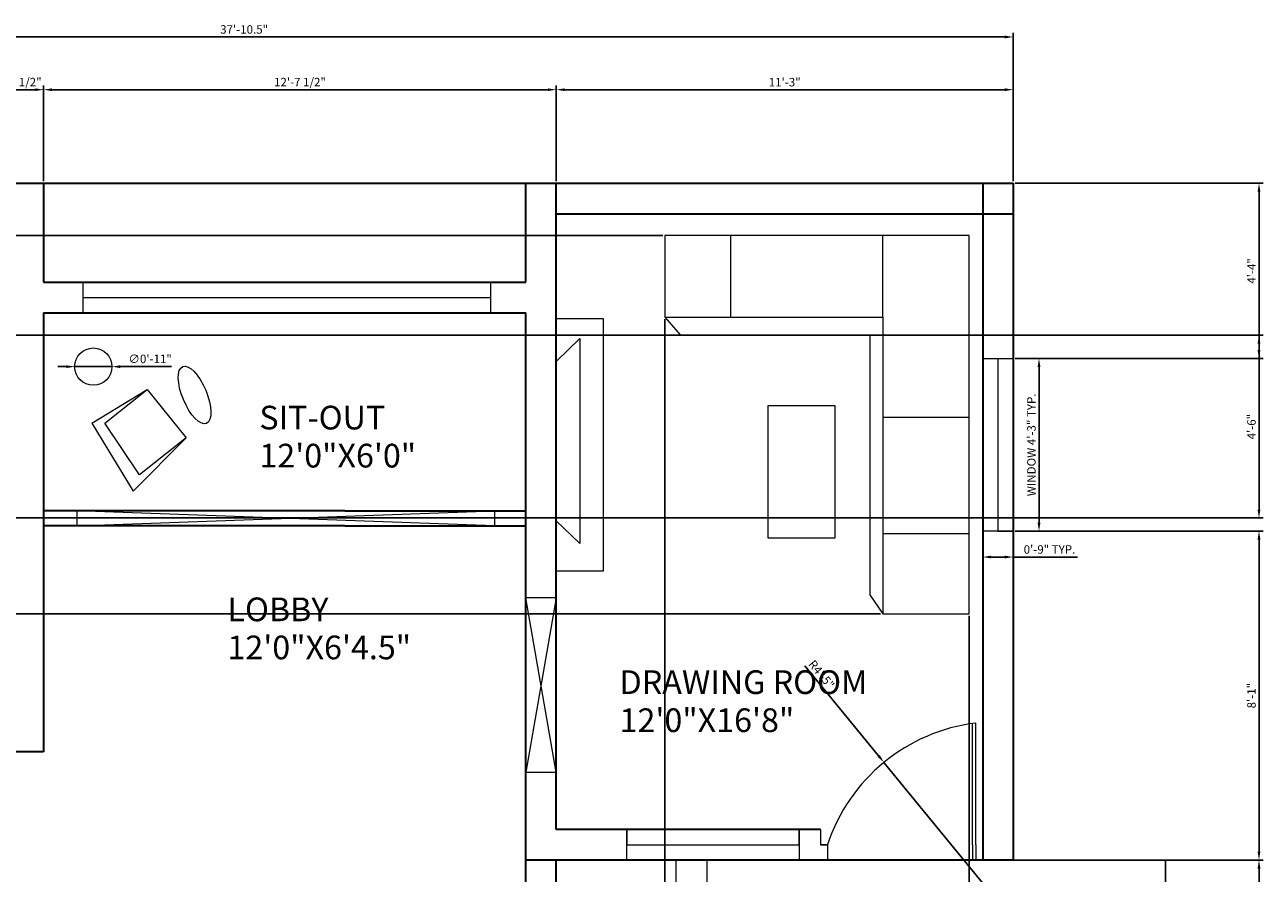
# Model space of a CAD drawing. Units: inches. Extents: x 1379 to 1989, y 1900 to 2397.
# Tile 3 of 3: x 1623 to 1989, y 2146 to 2397. Entities that reach past the tile are written whole.
import ezdxf

# ---------------------------------------------------------------- set-up
doc = ezdxf.new("R2010")
doc.units = ezdxf.units.IN
for name, color, linetype, lineweight in [('A-ANNO-DIMS', 2, 'Continuous', 18), ('A-AREA-IDEN', 7, 'Continuous', 18), ('A-DOOR', 3, 'Continuous', 18), ('A-FLOR', 7, 'Continuous', 25), ('A-FLOR-STRS', 7, 'Continuous', 18), ('A-FURN', 8, 'Continuous', 18), ('A-GLAZ', 4, 'Continuous', 18), ('A-WALL', 7, 'Continuous', 35)]:
    doc.layers.add(name, color=color, linetype=linetype, lineweight=lineweight)
doc.styles.get("Standard").update_dxf_attribs({"font": 'arial.ttf'})
doc.dimstyles.new('ISO-25', dxfattribs={"dimtxt": 2.5, "dimasz": 2.5, "dimexe": 1.25, "dimexo": 0.625, "dimtad": 1, "dimlunit": 3, "dimtxsty": 'Standard', "dimcen": 2.5, "dimadec": 0, "dimazin": 0, "dimtfac": 1, "dimtmove": 0, "dimatfit": 3, "dimfxl": 1, "dimarcsym": 0})

# ---------------------------------------------------------------- blocks, each defined once
blk = doc.blocks.new('*D6')
at = {"layer": 'A-ANNO-DIMS', "color": 0, "lineweight": -2, "transparency": 16777216}
for p, q in [((1460.41, 2350.93), (1460.41, 2394.79)), ((1462.91, 2393.54), (1912.41, 2393.54)), ((1914.91, 2350.93), (1914.91, 2394.79))]:
    blk.add_line(p, q, dxfattribs=at)
at = {"layer": 'A-ANNO-DIMS', "color": 0, "transparency": 16777216}
for points in [[(1462.91, 2393.95), (1462.91, 2393.12), (1460.41, 2393.54)], [(1912.41, 2393.95), (1912.41, 2393.12), (1914.91, 2393.54)]]:
    blk.add_solid(points, dxfattribs=at)
at = {"layer": 'Defpoints', "color": 0, "transparency": 16777216}
for p in [(1914.91, 2393.54), (1460.41, 2350.31), (1914.91, 2350.31)]:
    blk.add_point(p, dxfattribs=at)
at = {"layer": 'A-ANNO-DIMS', "color": 0, "transparency": 16777216, "insert": (1687.66, 2395.44), "char_height": 2.5, "attachment_point": 5}
blk.add_mtext('37\'-10.5"', dxfattribs=at)
blk = doc.blocks.new('WIN-51IN')
for p, q in [((0, 51), (9, 51)), ((4.5, 51), (4.5, 0)), ((9, 0), (0, 0)), ((4.5, 0), (9, 0))]:
    blk.add_line(p, q)
blk = doc.blocks.new('*D15')
at = {"layer": 'A-ANNO-DIMS', "color": 0, "lineweight": -2, "transparency": 16777216}
for p, q in [((1915.54, 2298.51), (1923.81, 2298.51)), ((1922.56, 2250.01), (1922.56, 2296.01)), ((1915.54, 2247.51), (1923.81, 2247.51))]:
    blk.add_line(p, q, dxfattribs=at)
at = {"layer": 'A-ANNO-DIMS', "color": 0, "transparency": 16777216}
for points in [[(1922.14, 2296.01), (1922.98, 2296.01), (1922.56, 2298.51)], [(1922.14, 2250.01), (1922.98, 2250.01), (1922.56, 2247.51)]]:
    blk.add_solid(points, dxfattribs=at)
at = {"layer": 'Defpoints', "color": 0, "transparency": 16777216}
for p in [(1914.91, 2298.51), (1922.56, 2298.51), (1914.91, 2247.51)]:
    blk.add_point(p, dxfattribs=at)
at = {"layer": 'A-ANNO-DIMS', "color": 0, "transparency": 16777216, "insert": (1920.64, 2273.01), "char_height": 2.5, "attachment_point": 5, "rotation": 90}
blk.add_mtext('WINDOW 4\'-3" TYP.', dxfattribs=at)
blk = doc.blocks.new('*D16')
at = {"layer": 'A-ANNO-DIMS', "color": 0, "lineweight": -2, "transparency": 16777216}
for p, q in [((1905.91, 2246.89), (1905.91, 2238.61)), ((1914.91, 2246.89), (1914.91, 2238.61)), ((1908.41, 2239.86), (1912.41, 2239.86)), ((1914.91, 2239.86), (1933.9, 2239.86))]:
    blk.add_line(p, q, dxfattribs=at)
at = {"layer": 'A-ANNO-DIMS', "color": 0, "transparency": 16777216}
for points in [[(1908.41, 2240.28), (1908.41, 2239.45), (1905.91, 2239.86)], [(1912.41, 2240.28), (1912.41, 2239.45), (1914.91, 2239.86)]]:
    blk.add_solid(points, dxfattribs=at)
at = {"layer": 'Defpoints', "color": 0, "transparency": 16777216}
for p in [(1905.91, 2247.51), (1914.91, 2247.51), (1914.91, 2239.86)]:
    blk.add_point(p, dxfattribs=at)
at = {"layer": 'A-ANNO-DIMS', "color": 0, "transparency": 16777216, "insert": (1925.65, 2241.77), "char_height": 2.5, "attachment_point": 5}
blk.add_mtext('0\'-9" TYP.', dxfattribs=at)
blk = doc.blocks.new('*D30')
at = {"layer": 'A-ANNO-DIMS', "color": 0, "lineweight": -2, "transparency": 16777216}
for p, q in [((1915.54, 2350.31), (1988.81, 2350.31)), ((1987.56, 2347.81), (1987.56, 2301.01)), ((1915.54, 2298.51), (1988.81, 2298.51))]:
    blk.add_line(p, q, dxfattribs=at)
at = {"layer": 'A-ANNO-DIMS', "color": 0, "transparency": 16777216}
for points in [[(1987.14, 2347.81), (1987.98, 2347.81), (1987.56, 2350.31)], [(1987.14, 2301.01), (1987.98, 2301.01), (1987.56, 2298.51)]]:
    blk.add_solid(points, dxfattribs=at)
at = {"layer": 'Defpoints', "color": 0, "transparency": 16777216}
for p in [(1914.91, 2350.31), (1914.91, 2298.51), (1987.56, 2298.51)]:
    blk.add_point(p, dxfattribs=at)
at = {"layer": 'A-ANNO-DIMS', "color": 0, "transparency": 16777216, "insert": (1985.69, 2324.41), "char_height": 2.5, "attachment_point": 5, "rotation": 90}
blk.add_mtext('4\'-4"', dxfattribs=at)
blk = doc.blocks.new('*D31')
at = {"layer": 'A-ANNO-DIMS', "color": 0, "lineweight": -2, "transparency": 16777216}
for p, q in [((1915.54, 2247.51), (1988.81, 2247.51)), ((1987.56, 2245.01), (1987.56, 2152.81)), ((1915.54, 2150.31), (1988.81, 2150.31))]:
    blk.add_line(p, q, dxfattribs=at)
at = {"layer": 'A-ANNO-DIMS', "color": 0, "transparency": 16777216}
for points in [[(1987.14, 2245.01), (1987.98, 2245.01), (1987.56, 2247.51)], [(1987.14, 2152.81), (1987.98, 2152.81), (1987.56, 2150.31)]]:
    blk.add_solid(points, dxfattribs=at)
at = {"layer": 'Defpoints', "color": 0, "transparency": 16777216}
for p in [(1914.91, 2247.51), (1914.91, 2150.31), (1987.56, 2150.31)]:
    blk.add_point(p, dxfattribs=at)
at = {"layer": 'A-ANNO-DIMS', "color": 0, "transparency": 16777216, "insert": (1985.66, 2198.91), "char_height": 2.5, "attachment_point": 5, "rotation": 90}
blk.add_mtext('8\'-1"', dxfattribs=at)
blk = doc.blocks.new('*D32')
at = {"layer": 'A-ANNO-DIMS', "color": 0, "lineweight": -2, "transparency": 16777216}
for p, q in [((1960.54, 2150.31), (1988.81, 2150.31)), ((1987.56, 1944.61), (1987.56, 2147.81)), ((1960.54, 1942.11), (1988.81, 1942.11))]:
    blk.add_line(p, q, dxfattribs=at)
at = {"layer": 'A-ANNO-DIMS', "color": 0, "transparency": 16777216}
for points in [[(1987.14, 2147.81), (1987.98, 2147.81), (1987.56, 2150.31)], [(1987.14, 1944.61), (1987.98, 1944.61), (1987.56, 1942.11)]]:
    blk.add_solid(points, dxfattribs=at)
at = {"layer": 'Defpoints', "color": 0, "transparency": 16777216}
for p in [(1959.91, 2150.31), (1987.56, 2150.31), (1959.91, 1942.11)]:
    blk.add_point(p, dxfattribs=at)
at = {"layer": 'A-ANNO-DIMS', "color": 0, "transparency": 16777216, "insert": (1985.68, 2046.21), "char_height": 2.5, "attachment_point": 5, "rotation": 90}
blk.add_mtext('17\'-4"', dxfattribs=at)
blk = doc.blocks.new('*D35')
at = {"layer": 'A-ANNO-DIMS', "color": 0, "lineweight": -2, "transparency": 16777216}
for p, q in [((1613.78, 2350.93), (1613.78, 2379.21)), ((1628.41, 2350.93), (1628.41, 2379.21)), ((1616.28, 2377.96), (1625.91, 2377.96))]:
    blk.add_line(p, q, dxfattribs=at)
at = {"layer": 'A-ANNO-DIMS', "color": 0, "transparency": 16777216}
for points in [[(1616.28, 2378.37), (1616.28, 2377.54), (1613.78, 2377.96)], [(1625.91, 2378.37), (1625.91, 2377.54), (1628.41, 2377.96)]]:
    blk.add_solid(points, dxfattribs=at)
at = {"layer": 'Defpoints', "color": 0, "transparency": 16777216}
for p in [(1628.41, 2377.96), (1613.78, 2350.31), (1628.41, 2350.31)]:
    blk.add_point(p, dxfattribs=at)
at = {"layer": 'A-ANNO-DIMS', "color": 0, "transparency": 16777216, "insert": (1621.1, 2379.88), "char_height": 2.5, "attachment_point": 5}
blk.add_mtext('1\'-2 1/2"', dxfattribs=at)
blk = doc.blocks.new('*D36')
at = {"layer": 'A-ANNO-DIMS', "color": 0, "lineweight": -2, "transparency": 16777216}
for p, q in [((1628.41, 2350.93), (1628.41, 2379.21)), ((1779.91, 2350.93), (1779.91, 2379.21)), ((1630.91, 2377.96), (1777.41, 2377.96))]:
    blk.add_line(p, q, dxfattribs=at)
at = {"layer": 'A-ANNO-DIMS', "color": 0, "transparency": 16777216}
for points in [[(1630.91, 2378.37), (1630.91, 2377.54), (1628.41, 2377.96)], [(1777.41, 2378.37), (1777.41, 2377.54), (1779.91, 2377.96)]]:
    blk.add_solid(points, dxfattribs=at)
at = {"layer": 'Defpoints', "color": 0, "transparency": 16777216}
for p in [(1779.91, 2377.96), (1628.41, 2350.31), (1779.91, 2350.31)]:
    blk.add_point(p, dxfattribs=at)
at = {"layer": 'A-ANNO-DIMS', "color": 0, "transparency": 16777216, "insert": (1704.16, 2379.88), "char_height": 2.5, "attachment_point": 5}
blk.add_mtext('12\'-7 1/2"', dxfattribs=at)
blk = doc.blocks.new('*D37')
at = {"layer": 'A-ANNO-DIMS', "color": 0, "lineweight": -2, "transparency": 16777216}
for p, q in [((1779.91, 2350.93), (1779.91, 2379.21)), ((1914.91, 2350.93), (1914.91, 2379.21)), ((1782.41, 2377.96), (1912.41, 2377.96))]:
    blk.add_line(p, q, dxfattribs=at)
at = {"layer": 'A-ANNO-DIMS', "color": 0, "transparency": 16777216}
for points in [[(1782.41, 2378.37), (1782.41, 2377.54), (1779.91, 2377.96)], [(1912.41, 2378.37), (1912.41, 2377.54), (1914.91, 2377.96)]]:
    blk.add_solid(points, dxfattribs=at)
at = {"layer": 'Defpoints', "color": 0, "transparency": 16777216}
for p in [(1914.91, 2377.96), (1779.91, 2350.31), (1914.91, 2350.31)]:
    blk.add_point(p, dxfattribs=at)
at = {"layer": 'A-ANNO-DIMS', "color": 0, "transparency": 16777216, "insert": (1847.41, 2379.86), "char_height": 2.5, "attachment_point": 5}
blk.add_mtext('11\'-3"', dxfattribs=at)
blk = doc.blocks.new('*D41')
at = {"layer": 'A-ANNO-DIMS', "color": 0, "lineweight": -2, "transparency": 16777216}
for p, q in [((1548.89, 2305.4), (1988.81, 2305.4)), ((1987.56, 2302.9), (1987.56, 2253.9)), ((1548.89, 2251.4), (1988.81, 2251.4))]:
    blk.add_line(p, q, dxfattribs=at)
at = {"layer": 'A-ANNO-DIMS', "color": 0, "transparency": 16777216}
for points in [[(1987.14, 2302.9), (1987.98, 2302.9), (1987.56, 2305.4)], [(1987.14, 2253.9), (1987.98, 2253.9), (1987.56, 2251.4)]]:
    blk.add_solid(points, dxfattribs=at)
at = {"layer": 'Defpoints', "color": 0, "transparency": 16777216}
for p in [(1548.27, 2305.4), (1548.27, 2251.4), (1987.56, 2251.4)]:
    blk.add_point(p, dxfattribs=at)
at = {"layer": 'A-ANNO-DIMS', "color": 0, "transparency": 16777216, "insert": (1985.66, 2278.4), "char_height": 2.5, "attachment_point": 5, "rotation": 90}
blk.add_mtext('4\'-6"', dxfattribs=at)
blk = doc.blocks.new('*D42')
at = {"layer": 'A-ANNO-DIMS', "color": 0, "lineweight": -2, "transparency": 16777216}
for p, q in [((1811.97, 2310.14), (1811.97, 1900.58)), ((1901.92, 2222.46), (1901.92, 1900.58)), ((1814.47, 1901.83), (1899.42, 1901.83))]:
    blk.add_line(p, q, dxfattribs=at)
at = {"layer": 'A-ANNO-DIMS', "color": 0, "transparency": 16777216}
for points in [[(1814.47, 1902.24), (1814.47, 1901.41), (1811.97, 1901.83)], [(1899.42, 1902.24), (1899.42, 1901.41), (1901.92, 1901.83)]]:
    blk.add_solid(points, dxfattribs=at)
at = {"layer": 'Defpoints', "color": 0, "transparency": 16777216}
for p in [(1811.97, 2310.77), (1901.92, 2223.09), (1901.92, 1901.83)]:
    blk.add_point(p, dxfattribs=at)
at = {"layer": 'A-ANNO-DIMS', "color": 0, "transparency": 16777216, "insert": (1856.94, 1903.73), "char_height": 2.5, "attachment_point": 5}
blk.add_mtext('7\'-6"', dxfattribs=at)
blk = doc.blocks.new('*D43')
at = {"layer": 'A-ANNO-DIMS', "color": 0, "lineweight": -2, "transparency": 16777216}
for p, q in [((1811.35, 2334.84), (1380.86, 2334.84)), ((1382.11, 2332.34), (1382.11, 2225.59)), ((1875.73, 2223.09), (1380.86, 2223.09))]:
    blk.add_line(p, q, dxfattribs=at)
at = {"layer": 'A-ANNO-DIMS', "color": 0, "transparency": 16777216}
for points in [[(1381.7, 2332.34), (1382.53, 2332.34), (1382.11, 2334.84)], [(1381.7, 2225.59), (1382.53, 2225.59), (1382.11, 2223.09)]]:
    blk.add_solid(points, dxfattribs=at)
at = {"layer": 'Defpoints', "color": 0, "transparency": 16777216}
for p in [(1811.97, 2334.84), (1382.11, 2223.09), (1876.36, 2223.09)]:
    blk.add_point(p, dxfattribs=at)
at = {"layer": 'A-ANNO-DIMS', "color": 0, "transparency": 16777216, "insert": (1380.21, 2278.96), "char_height": 2.5, "attachment_point": 5, "rotation": 90}
blk.add_mtext('9\'-4"', dxfattribs=at)
blk = doc.blocks.new('*D44')
at = {"layer": 'A-ANNO-DIMS', "color": 0, "lineweight": -2, "transparency": 16777216}
for p, q in [((1853.31, 2207.74), (1875.14, 2181.12)), ((1910.32, 2138.22), (1876.73, 2179.19))]:
    blk.add_line(p, q, dxfattribs=at)
at = {"layer": 'A-ANNO-DIMS', "color": 0, "transparency": 16777216}
blk.add_solid([(1875.47, 2181.38), (1874.82, 2180.85), (1876.73, 2179.19)], dxfattribs=at)
at = {"layer": 'Defpoints', "color": 0, "transparency": 16777216}
for p in [(1876.73, 2179.19), (1910.32, 2138.22)]:
    blk.add_point(p, dxfattribs=at)
at = {"layer": 'A-ANNO-DIMS', "color": 0, "transparency": 16777216, "insert": (1858.04, 2204.97), "char_height": 2.5, "attachment_point": 5, "rotation": 309.3523}
blk.add_mtext('R4\'-5"', dxfattribs=at)
blk = doc.blocks.new('*D51')
at = {"layer": 'A-ANNO-DIMS', "color": 0, "lineweight": -2, "transparency": 16777216}
for p, q in [((1635.07, 2296.12), (1632.57, 2296.12)), ((1637.57, 2296.12), (1648.6, 2296.12)), ((1666.16, 2296.12), (1651.1, 2296.12))]:
    blk.add_line(p, q, dxfattribs=at)
at = {"layer": 'A-ANNO-DIMS', "color": 0, "transparency": 16777216}
for points in [[(1635.07, 2296.54), (1635.07, 2295.7), (1637.57, 2296.12)], [(1651.1, 2296.54), (1651.1, 2295.7), (1648.6, 2296.12)]]:
    blk.add_solid(points, dxfattribs=at)
at = {"layer": 'Defpoints', "color": 0, "transparency": 16777216}
for p in [(1637.57, 2296.12), (1648.6, 2296.12)]:
    blk.add_point(p, dxfattribs=at)
at = {"layer": 'A-ANNO-DIMS', "color": 0, "transparency": 16777216, "insert": (1659.88, 2298.09), "char_height": 2.5, "attachment_point": 5, "rotation": 0.003}
blk.add_mtext('∅0\'-11"', dxfattribs=at)

msp = doc.modelspace()

# ---------------------------------------------------------------- linework, layer by layer
at = {"layer": 'A-DOOR'}
for p, q in [((1902.91, 2154.808), (1902.91, 2190.676)), ((1903.91, 2154.808), (1903.91, 2190.808)), ((1858.009, 2159.308), (1858.009, 2154.808)), ((1905.91, 2159.308), (1905.91, 2154.808)), ((1858.009, 2154.808), (1860.009, 2154.808)), ((1860.009, 2154.808), (1858.009, 2154.808)), ((1860.009, 2154.808), (1860.009, 2150.308)), ((1902.91, 2154.808), (1902.91, 2150.308)), ((1903.91, 2154.808), (1903.91, 2150.308))]:
    msp.add_line(p, q, dxfattribs=at)
msp.add_arc((1910.322, 2138.221), 52.977, 96.95114, 161.75354, dxfattribs=at)
at = {"layer": 'A-FLOR'}
for p, q in [((1959.91, 2150.308), (1914.91, 2150.308)), ((1959.91, 2049.582), (1959.91, 2150.308))]:
    msp.add_line(p, q, dxfattribs=at)
at = {"layer": 'A-FLOR-STRS'}
for p, q in [((1815.368, 2046.02), (1815.368, 2150.308)), ((1824.368, 2150.308), (1824.368, 2045.838))]:
    msp.add_line(p, q, dxfattribs=at)
at = {"layer": 'A-FURN'}
for p, q in [((1811.97, 2334.839), (1811.97, 2310.77)), ((1901.918, 2334.839), (1811.97, 2334.839)), ((1831.376, 2334.839), (1831.376, 2310.77)), ((1876.359, 2310.77), (1876.359, 2334.839)), ((1901.918, 2223.089), (1901.918, 2334.839)), ((1779.91, 2310.332), (1793.758, 2310.332)), ((1793.758, 2310.332), (1793.758, 2235.684)), ((1811.97, 2310.77), (1876.359, 2310.77)), ((1811.97, 2310.77), (1816.463, 2305.541)), ((1831.376, 2310.77), (1876.359, 2310.77)), ((1876.359, 2310.77), (1876.359, 2223.089)), ((1779.91, 2297.612), (1786.829, 2304.448)), ((1786.829, 2304.448), (1786.829, 2243.831)), ((1816.463, 2305.541), (1872.587, 2305.541)), ((1872.587, 2305.541), (1872.587, 2228.737)), ((1642.639, 2279.436), (1659.035, 2289.416)), ((1646.514, 2279.436), (1659.035, 2289.416)), ((1659.035, 2289.416), (1670.494, 2275.041)), ((1876.359, 2281.159), (1901.918, 2281.159)), ((1642.639, 2279.436), (1654.881, 2259.324)), ((1656.782, 2264.111), (1646.514, 2279.436)), ((1654.881, 2259.324), (1670.494, 2275.041)), ((1670.494, 2275.041), (1656.782, 2264.111)), ((1786.829, 2243.831), (1779.91, 2250.56)), ((1876.359, 2246.795), (1901.918, 2246.795)), ((1793.758, 2235.684), (1779.91, 2235.684)), ((1872.587, 2228.737), (1876.359, 2223.089)), ((1876.359, 2223.089), (1901.918, 2223.089))]:
    msp.add_line(p, q, dxfattribs=at)
msp.add_lwpolyline([(1842.556, 2284.681), (1862.194, 2284.681), (1862.194, 2245.428), (1842.556, 2245.428)], close=True, dxfattribs=at)
msp.add_circle((1643.086, 2296.12), 5.515, dxfattribs=at)
msp.add_ellipse((1673.02, 2287.75), major_axis=(3.501, -8.385), ratio=0.3949454, dxfattribs=at)
at = {"layer": 'A-GLAZ'}
for p, q in [((1639.98, 2321.038), (1639.98, 2312.038)), ((1760.445, 2321.038), (1760.445, 2312.038)), ((1639.98, 2316.538), (1760.445, 2316.538)), ((1638.173, 2253.538), (1638.173, 2249.038)), ((1638.173, 2249.038), (1761.604, 2253.538)), ((1761.604, 2249.038), (1638.173, 2253.538)), ((1761.604, 2253.538), (1761.604, 2249.038)), ((1779.91, 2227.839), (1770.91, 2227.839)), ((1779.91, 2227.839), (1770.91, 2176.31)), ((1779.91, 2176.31), (1770.91, 2227.839)), ((1770.91, 2176.31), (1779.91, 2176.31)), ((1770.91, 2176.31), (1779.91, 2176.31)), ((1800.714, 2159.308), (1800.714, 2154.808))]:
    msp.add_line(p, q, dxfattribs=at)
at = {"layer": 'A-WALL'}
for p, q in [((1460.41, 2350.308), (1628.41, 2350.308)), ((1628.41, 2350.308), (1628.41, 2321.038)), ((1628.41, 2350.308), (1760.41, 2350.308)), ((1760.41, 2350.308), (1779.91, 2350.308)), ((1770.91, 2350.308), (1914.91, 2350.308)), ((1770.91, 2321.038), (1770.91, 2350.308)), ((1779.91, 2159.308), (1779.91, 2350.308)), ((1905.91, 2350.308), (1905.91, 2150.308)), ((1914.91, 2350.308), (1914.91, 2150.308)), ((1779.91, 2341.308), (1914.91, 2341.308)), ((1628.41, 2321.038), (1770.91, 2321.038)), ((1628.41, 2312.038), (1770.91, 2312.038)), ((1628.41, 2312.038), (1628.41, 2182.308)), ((1770.91, 2040.582), (1770.91, 2312.038)), ((1717.462, 2253.538), (1628.41, 2253.538)), ((1717.462, 2253.538), (1770.91, 2253.538)), ((1717.462, 2249.038), (1628.41, 2249.038)), ((1717.462, 2249.038), (1770.91, 2249.038)), ((1628.41, 2182.308), (1613.41, 2182.308)), ((1858.009, 2159.308), (1779.91, 2159.308)), ((1914.91, 2150.308), (1770.91, 2150.308)), ((1779.91, 2049.582), (1779.91, 2150.308))]:
    msp.add_line(p, q, dxfattribs=at)

# ---------------------------------------------------------------- block references
at = {"layer": 'A-GLAZ'}
msp.add_blockref('WIN-51IN', (1905.91, 2247.514), dxfattribs=at)
at = {"layer": 'A-GLAZ', "rotation": 89.99999999999955}
msp.add_blockref('WIN-51IN', (1851.715, 2150.308), dxfattribs=at)

# ---------------------------------------------------------------- texts
at = {"layer": 'A-AREA-IDEN'}
for s, p in [('SIT-OUT', (1692.153, 2277.567)), ('12\'0"X6\'0"', (1692.153, 2266.322)), ('LOBBY', (1682.716, 2220.9)), ('12\'0"X6\'4.5"', (1682.716, 2209.656)), ('DRAWING ROOM', (1798.594, 2199.391)), ('12\'0"X16\'8"', (1798.594, 2188.146))]:
    msp.add_text(s, height=7, dxfattribs=at).set_placement(p)

# ---------------------------------------------------------------- dimensions: what is measured, and where the dimension line sits
at = {"layer": 'A-ANNO-DIMS'}
for base, p1, p2, override, picture, middle in [((1914.91, 2393.536), (1460.41, 2350.308), (1914.91, 2350.308), {"dimclrd": 0, "dimclre": 0, "dimclrt": 0}, '*D6', (1687.66, 2395.438)), ((1628.41, 2377.958), (1613.78, 2350.308), (1628.41, 2350.308), {"dimdec": 1, "dimlfac": 1, "dimrnd": 0, "dimzin": 1, "dimdsep": 46, "dimlunit": 4, "dimfrac": 2}, '*D35', (1621.095, 2379.875)), ((1779.91, 2377.958), (1628.41, 2350.308), (1779.91, 2350.308), {"dimdec": 1, "dimlfac": 1, "dimrnd": 0, "dimzin": 1, "dimdsep": 46, "dimlunit": 4, "dimfrac": 2}, '*D36', (1704.16, 2379.875)), ((1914.91, 2377.958), (1779.91, 2350.308), (1914.91, 2350.308), {"dimdec": 1, "dimlfac": 1, "dimrnd": 0, "dimzin": 1, "dimdsep": 46, "dimlunit": 4, "dimfrac": 2}, '*D37', (1847.41, 2379.86)), ((1901.918, 1901.828), (1811.97, 2310.77), (1901.918, 2223.089), {"dimdec": 1, "dimlfac": 1, "dimrnd": 0, "dimzin": 1, "dimdsep": 46, "dimlunit": 4, "dimfrac": 2}, '*D42', (1856.944, 1903.729))]:
    dim = msp.add_linear_dim(base=base, p1=p1, p2=p2, dimstyle='ISO-25', override=override, dxfattribs=at)
    dim.commit()
    dim.dimension.update_dxf_attribs({"geometry": picture, "text_midpoint": middle})
for base, p1, p2, picture, middle in [((1987.56, 2298.515), (1914.91, 2350.308), (1914.91, 2298.515), '*D30', (1985.685, 2324.411)), ((1382.1123, 2223.0887), (1811.9703, 2334.8388), (1876.3593, 2223.0887), '*D43', (1380.2108, 2278.9637)), ((1987.56, 2251.398), (1548.266, 2305.398), (1548.266, 2251.398), '*D41', (1985.659, 2278.398)), ((1987.56, 2150.308), (1914.91, 2247.515), (1914.91, 2150.308), '*D31', (1985.659, 2198.911)), ((1987.56, 2150.308), (1959.91, 1942.11), (1959.91, 2150.308), '*D32', (1985.68, 2046.209))]:
    dim = msp.add_linear_dim(base=base, p1=p1, p2=p2, angle=90, dimstyle='ISO-25', override={"dimdec": 1, "dimlfac": 1, "dimrnd": 0, "dimzin": 1, "dimdsep": 46, "dimlunit": 4, "dimfrac": 2}, dxfattribs=at)
    dim.commit()
    dim.dimension.update_dxf_attribs({"geometry": picture, "text_midpoint": middle})
dim = msp.add_diameter_dim_2p(p1=(1637.571, 2296.119), p2=(1648.601, 2296.12), dimstyle='ISO-25', override={"dimdec": 1, "dimlfac": 1, "dimrnd": 0, "dimzin": 1, "dimdsep": 46, "dimlunit": 4, "dimfrac": 2}, dxfattribs=at)
dim.commit()
dim.dimension.update_dxf_attribs({"geometry": '*D51', "text_midpoint": (1659.88, 2296.121), "dimtype": 163})
dim = msp.add_linear_dim(base=(1922.56, 2298.515), p1=(1914.91, 2247.515), p2=(1914.91, 2298.515), angle=90, text='WINDOW <> TYP.', dimstyle='ISO-25', override={"dimdec": 1, "dimlfac": 1, "dimrnd": 0, "dimzin": 1, "dimdsep": 46, "dimlunit": 4, "dimfrac": 2}, dxfattribs=at)
dim.commit()
dim.dimension.update_dxf_attribs({"geometry": '*D15', "text_midpoint": (1920.641, 2273.015)})
dim = msp.add_linear_dim(base=(1914.91, 2239.865), p1=(1905.91, 2247.515), p2=(1914.91, 2247.515), text='<> TYP.', dimstyle='ISO-25', override={"dimdec": 1, "dimlfac": 1, "dimrnd": 0, "dimzin": 1, "dimdsep": 46, "dimlunit": 4, "dimfrac": 2}, dxfattribs=at)
dim.commit()
dim.dimension.update_dxf_attribs({"geometry": '*D16', "text_midpoint": (1925.655, 2241.766)})
dim = msp.add_radius_dim(center=(1910.322, 2138.221), mpoint=(1876.73, 2179.185), dimstyle='ISO-25', override={"dimdec": 1, "dimlfac": 1, "dimrnd": 0, "dimzin": 1, "dimdsep": 46, "dimlunit": 4, "dimfrac": 2}, dxfattribs=at)
dim.commit()
dim.dimension.update_dxf_attribs({"geometry": '*D44', "text_midpoint": (1856.575, 2203.764), "dimtype": 164})

doc.saveas('drawing.dxf')
